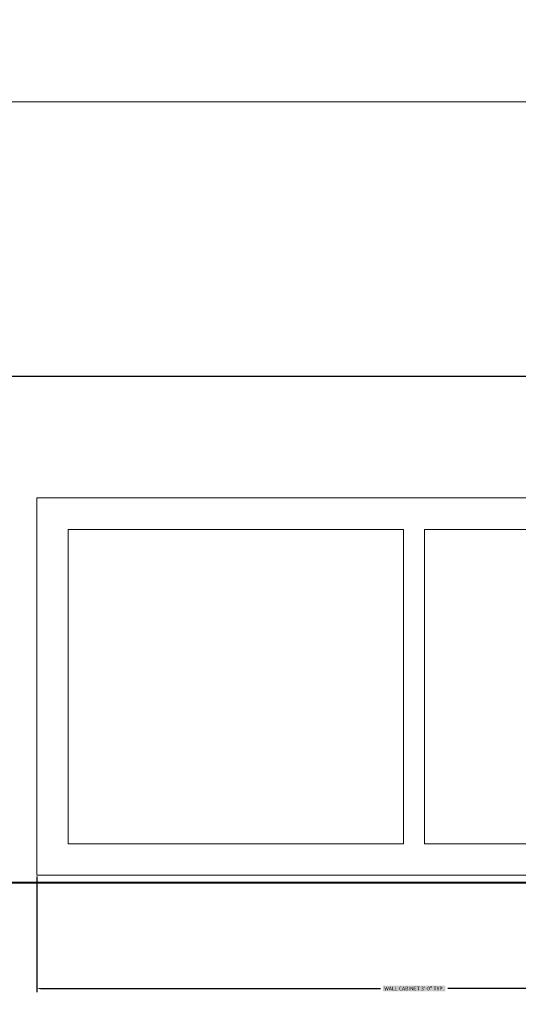
# Model space of a CAD drawing. Units: inches. Extents: x -301 to 715, y -607 to 364.
# Tile 69 of 141: x -171 to -147, y -73 to -26. Entities that reach past the tile are written whole.
import ezdxf

# ---------------------------------------------------------------- set-up
doc = ezdxf.new("R2010")
doc.units = ezdxf.units.IN
doc.header["$MEASUREMENT"] = 0
for name, color, linetype, lineweight in [('A-ANNO-DIMS', 2, 'Continuous', 18), ('A-FLOR-CASE', 8, 'Continuous', 18), ('A-FURN', 8, 'Continuous', 18), ('A-WALL', 3, 'Continuous', 40)]:
    doc.layers.add(name, color=color, linetype=linetype, lineweight=lineweight)
doc.styles.get("Standard").update_dxf_attribs({"font": 'arial.ttf'})
doc.dimstyles.get("Standard").update_dxf_attribs({"dimtxt": 0.18, "dimasz": 0.18, "dimexe": 0.18, "dimexo": 0.0625, "dimgap": 0.09, "dimtad": 0, "dimtih": 1, "dimtoh": 1, "dimdec": 1, "dimzin": 0, "dimdsep": 46, "dimlunit": 4, "dimtxsty": 'Standard', "dimcen": 0.09, "dimclrd": 3, "dimclre": 4, "dimclrt": 6, "dimadec": 0, "dimazin": 0, "dimtfac": 1, "dimtdec": 1, "dimtofl": 0, "dimtmove": 0, "dimatfit": 3, "dimfxl": 1, "dimtfill": 2, "dimtfillclr": 51, "dimtolj": 1, "dimtzin": 0, "dimarcsym": 0})

# ---------------------------------------------------------------- blocks, each defined once
blk = doc.blocks.new('Bed - Queen')
blk.add_line((0, -80.00003), (0, 0))
blk = doc.blocks.new('Wall Cabinet - 18 x 36 in front')
for p, q in [((17.5, -1.5), (17.5, -16.5)), ((18.5, -16.5), (18.5, -1.5))]:
    blk.add_line(p, q)
blk.add_lwpolyline([(0, -18), (0, 0), (36, 0), (36, -18)], close=True)
for points in [[(17.5, -16.5), (1.5, -16.5), (1.5, -1.5), (17.5, -1.5)], [(18.5, -1.5), (34.5, -1.5), (34.5, -16.5), (18.5, -16.5)]]:
    blk.add_lwpolyline(points)
blk = doc.blocks.new('*D56')
at = {"layer": 'A-ANNO-DIMS', "color": 0, "lineweight": -2, "transparency": 16777216}
for p, q in [((-195.541, 65.682), (-172.295, 65.682)), ((-172.475, 60.682), (-172.475, 0.778)), ((-172.475, -62.318), (-172.475, -2.414)), ((-195.541, -67.318), (-172.295, -67.318))]:
    blk.add_line(p, q, dxfattribs=at)
at = {"layer": 'A-ANNO-DIMS', "color": 0, "transparency": 16777216}
for points in [[(-173.308, 60.682), (-171.641, 60.682), (-172.475, 65.682)], [(-173.308, -62.318), (-171.641, -62.318), (-172.475, -67.318)]]:
    blk.add_solid(points, dxfattribs=at)
at = {"layer": 'Defpoints', "color": 0, "transparency": 16777216}
for p in [(-195.603, 65.682), (-172.475, 65.682), (-195.603, -67.318)]:
    blk.add_point(p, dxfattribs=at)
at = {"layer": 'A-ANNO-DIMS', "color": 0, "transparency": 16777216, "insert": (-172.475, -0.818), "char_height": 3, "attachment_point": 5, "bg_fill": 1, "box_fill_scale": 1.25, "bg_fill_color": 51, "bg_fill_transparency": 0}
blk.add_mtext('\\A1;11\'-1"', dxfattribs=at)
blk = doc.blocks.new('*D57')
at = {"layer": 'A-ANNO-DIMS', "color": 0, "lineweight": -2, "transparency": 16777216}
for p, q in [((-195.603, -67.255), (-195.603, -42.99)), ((-190.603, -43.17), (-126.098, -43.17)), ((-56.603, -43.17), (-121.109, -43.17)), ((-51.603, -67.255), (-51.603, -42.99))]:
    blk.add_line(p, q, dxfattribs=at)
at = {"layer": 'A-ANNO-DIMS', "color": 0, "transparency": 16777216}
for points in [[(-190.603, -42.336), (-190.603, -44.003), (-195.603, -43.17)], [(-56.603, -42.336), (-56.603, -44.003), (-51.603, -43.17)]]:
    blk.add_solid(points, dxfattribs=at)
at = {"layer": 'Defpoints', "color": 0, "transparency": 16777216}
for p in [(-51.603, -43.17), (-195.603, -67.318), (-51.603, -67.318)]:
    blk.add_point(p, dxfattribs=at)
at = {"layer": 'A-ANNO-DIMS', "color": 0, "transparency": 16777216, "insert": (-123.603, -43.17), "char_height": 3, "attachment_point": 5, "bg_fill": 1, "box_fill_scale": 1.25, "bg_fill_color": 51, "bg_fill_transparency": 0}
blk.add_mtext("\\A1;12'", dxfattribs=at)
blk = doc.blocks.new('*D120')
at = {"layer": 'A-ANNO-DIMS', "color": 4, "lineweight": -2, "transparency": 16777216}
for p, q in [((-170.223, -67.046), (-170.223, -72.563)), ((-134.223, -67.046), (-134.223, -72.563))]:
    blk.add_line(p, q, dxfattribs=at)
at = {"layer": 'A-ANNO-DIMS', "color": 3, "lineweight": -2, "transparency": 16777216}
for p, q in [((-170.043, -72.383), (-153.822, -72.383)), ((-134.403, -72.383), (-150.623, -72.383))]:
    blk.add_line(p, q, dxfattribs=at)
at = {"layer": 'A-ANNO-DIMS', "color": 3, "transparency": 16777216}
for points in [[(-170.043, -72.353), (-170.043, -72.413), (-170.223, -72.383)], [(-134.403, -72.353), (-134.403, -72.413), (-134.223, -72.383)]]:
    blk.add_solid(points, dxfattribs=at)
at = {"layer": 'Defpoints', "color": 0, "transparency": 16777216}
for p in [(-170.223, -66.983), (-134.223, -66.983), (-134.223, -72.383)]:
    blk.add_point(p, dxfattribs=at)
at = {"layer": 'A-ANNO-DIMS', "color": 6, "transparency": 16777216, "insert": (-152.223, -72.383), "char_height": 0.18, "attachment_point": 5, "bg_fill": 1, "box_fill_scale": 1.25, "bg_fill_color": 51, "bg_fill_transparency": 0}
blk.add_mtext('\\A1;WALL CABINET 3\'-0" TYP.', dxfattribs=at)
blk = doc.blocks.new('*D151')
at = {"layer": 'A-ANNO-DIMS', "color": 4, "lineweight": -2, "transparency": 16777216}
for p, q in [((-204.603, -223.755), (-204.603, 359.612)), ((-45.603, -214.755), (-45.603, 359.612))]:
    blk.add_line(p, q, dxfattribs=at)
at = {"layer": 'A-ANNO-DIMS', "color": 3, "lineweight": -2, "transparency": 16777216}
for p, q in [((-204.423, 359.432), (-125.494, 359.432)), ((-45.783, 359.432), (-124.713, 359.432))]:
    blk.add_line(p, q, dxfattribs=at)
at = {"layer": 'A-ANNO-DIMS', "color": 3, "transparency": 16777216}
for points in [[(-204.423, 359.462), (-204.423, 359.402), (-204.603, 359.432)], [(-45.783, 359.462), (-45.783, 359.402), (-45.603, 359.432)]]:
    blk.add_solid(points, dxfattribs=at)
at = {"layer": 'Defpoints', "color": 0, "transparency": 16777216}
for p in [(-45.603, 359.432), (-45.603, -214.818), (-204.603, -223.818)]:
    blk.add_point(p, dxfattribs=at)
at = {"layer": 'A-ANNO-DIMS', "color": 6, "transparency": 16777216, "insert": (-125.103, 359.432), "char_height": 0.18, "attachment_point": 5, "bg_fill": 1, "box_fill_scale": 1.25, "bg_fill_color": 51, "bg_fill_transparency": 0}
blk.add_mtext('\\A1;13\'-3"', dxfattribs=at)

msp = doc.modelspace()

# ---------------------------------------------------------------- linework, layer by layer
at = {"layer": 'A-WALL'}
msp.add_line((-195.603, -67.318), (-51.603, -67.318), dxfattribs=at)

# ---------------------------------------------------------------- block references
at = {"layer": 'A-FLOR-CASE'}
msp.add_blockref('Wall Cabinet - 18 x 36 in front', (-170.223, -48.983), dxfattribs=at)
at = {"layer": 'A-FURN', "xscale": 0.8856750462000775, "yscale": 0.8856750462000775, "zscale": 0.8856750462000775, "rotation": 90}
msp.add_blockref('Bed - Queen', (-195.207, -30.095), dxfattribs=at)

# ---------------------------------------------------------------- dimensions: what is measured, and where the dimension line sits
at = {"layer": 'A-ANNO-DIMS'}
for base, p1, p2, override, picture, middle in [((-45.603, 359.432), (-204.603, -223.818), (-45.603, -214.818), {"dimdec": 1, "dimlfac": 1, "dimrnd": 0, "dimzin": 1, "dimdsep": 46, "dimlunit": 4, "dimfrac": 2}, '*D151', (-125.103, 359.432)), ((-51.603, -43.17), (-195.603, -67.318), (-51.603, -67.318), {"dimtxt": 3, "dimasz": 5, "dimclrd": 0, "dimclre": 0, "dimclrt": 0}, '*D57', (-123.603, -43.17))]:
    dim = msp.add_linear_dim(base=base, p1=p1, p2=p2, dimstyle='Standard', override=override, dxfattribs=at)
    dim.commit()
    dim.dimension.update_dxf_attribs({"geometry": picture, "text_midpoint": middle})
dim = msp.add_linear_dim(base=(-172.475, 65.682), p1=(-195.603, -67.318), p2=(-195.603, 65.682), angle=90, dimstyle='Standard', override={"dimtxt": 3, "dimasz": 5, "dimclrd": 0, "dimclre": 0, "dimclrt": 0}, dxfattribs=at)
dim.commit()
dim.dimension.update_dxf_attribs({"geometry": '*D56', "text_midpoint": (-172.475, -0.818)})
dim = msp.add_linear_dim(base=(-134.223, -72.383), p1=(-170.223, -66.983), p2=(-134.223, -66.983), text='WALL CABINET <> TYP.', dimstyle='Standard', override={"dimdec": 1, "dimlfac": 1, "dimrnd": 0, "dimzin": 1, "dimdsep": 46, "dimlunit": 4, "dimfrac": 2}, dxfattribs=at)
dim.commit()
dim.dimension.update_dxf_attribs({"geometry": '*D120', "text_midpoint": (-152.223, -72.383)})

doc.saveas('drawing.dxf')
